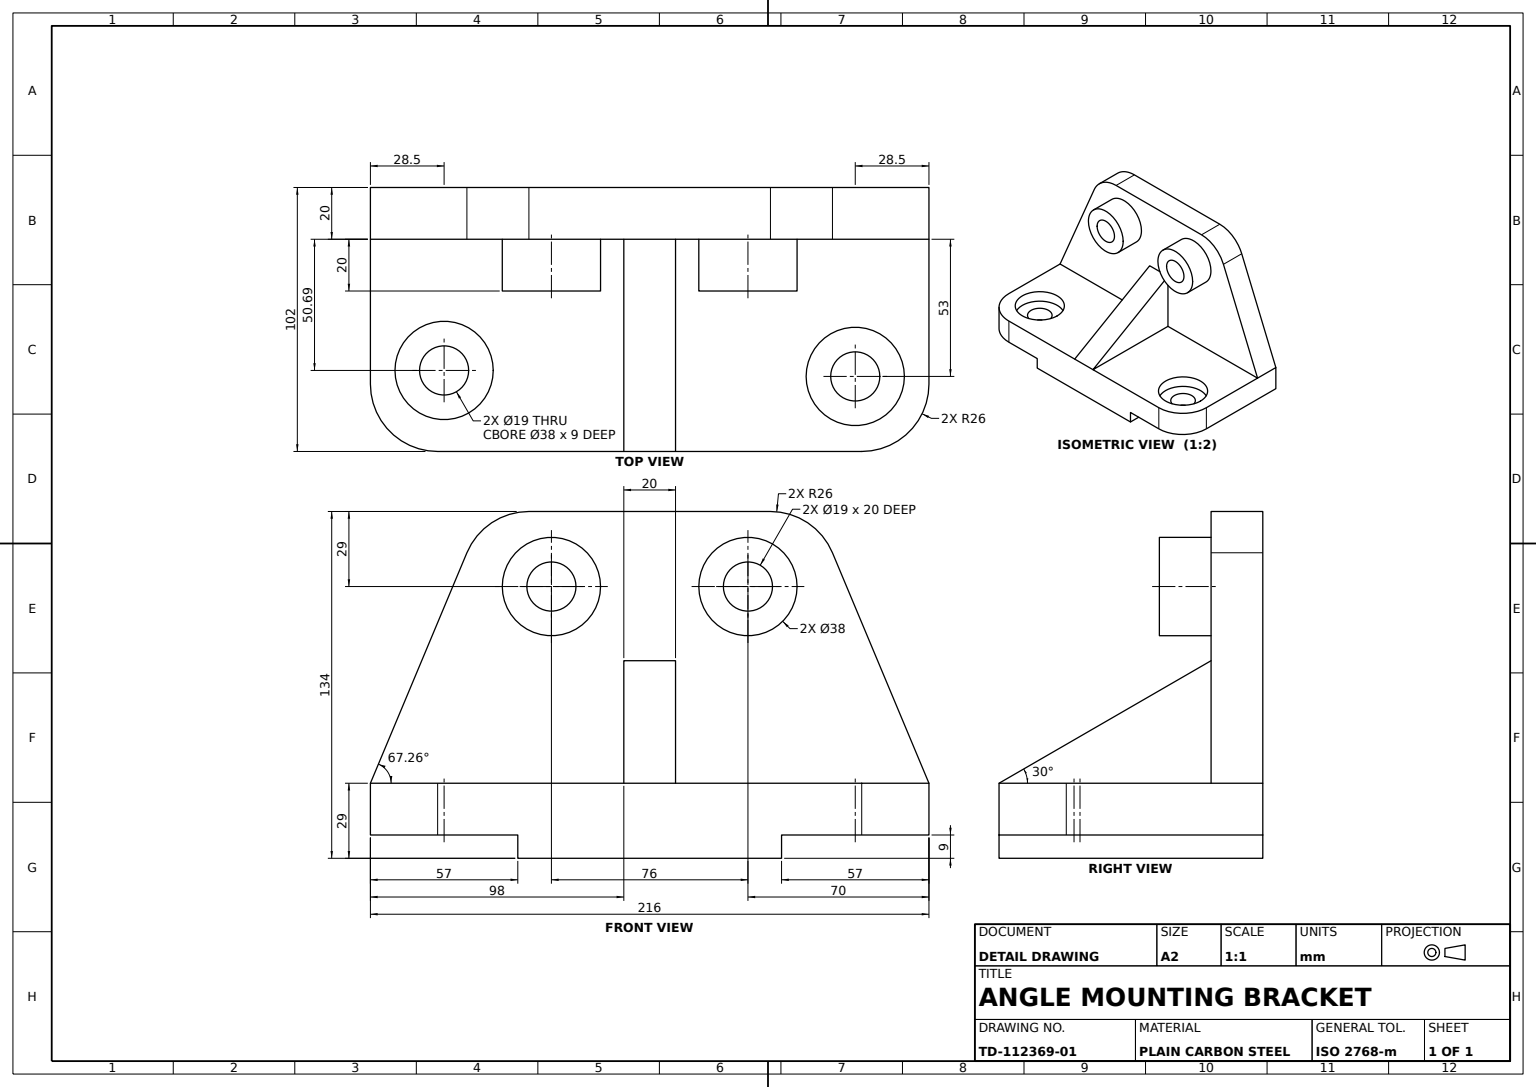
from build123d import *

# Parameters (mm, degrees)
BASE_PLATE_DEPTH                = 102
UPRIGHT_PLATE_DEPTH             = 20
UPRIGHT_BOSS_1_PROFILE_R        = 19
UPRIGHT_BOSS_1_PROFILE_R_2      = 9.5
UPRIGHT_BOSS_1_DEPTH            = 20
UPRIGHT_BOSS_2_PROFILE_R        = 19
UPRIGHT_BOSS_2_PROFILE_R_2      = 9.5
UPRIGHT_BOSS_2_DEPTH            = 20
BASE_POCKET_1_PROFILE_R         = 19
BASE_POCKET_1_DEPTH             = 9
MOUNTING_HOLE_1_PROFILE_R       = 9.5
MOUNTING_HOLE_1_DEPTH           = 265.680940001
BASE_POCKET_2_PROFILE_R         = 19
BASE_POCKET_2_DEPTH             = 9
MOUNTING_HOLE_2_PROFILE_R       = 9.5
MOUNTING_HOLE_2_DEPTH           = 265.680940001
UPRIGHT_CORNER_FILLET_R26_1_R   = 26
UPRIGHT_CORNER_FILLET_R26_2_R   = 26
BASE_CORNER_FILLETS_R26_R       = 26
GUSSET_RIB_REACH                = 196.147
GUSSET_RIB_PROFILE_30DEG_WALL_W = 484.979147418
GUSSET_RIB_PROFILE_30DEG_WALL_H = 20


with BuildPart() as part:
    # Base Plate Profile → Base Plate (new body)
    with BuildSketch(Plane(origin=(0, 0, 0), x_dir=(0, 0, -1), z_dir=(1, 0, 0))):
        Polygon((0, 0), (57, 0), (57, -9), (159, -9), (159, 0), (216, 0), (216, 20), (0, 20), align=None)
    extrude(amount=BASE_PLATE_DEPTH)

    # Upright Plate Profile → Upright Plate (add)
    with BuildSketch(Plane(origin=(0, 0, 0), x_dir=(0, 0, -1), z_dir=(1, 0, 0))):
        Polygon((0, 20), (216, 20), (172, 125), (44, 125), align=None)
    extrude(amount=UPRIGHT_PLATE_DEPTH)

    # Upright Boss 1 Profile → Upright Boss 1 (add)
    with BuildSketch(Plane(origin=(20, 0, 0), x_dir=(0, 0, -1), z_dir=(1, 0, 0))):
        with Locations((70, 96)):
            Circle(UPRIGHT_BOSS_1_PROFILE_R)
        with Locations((70, 96)):
            Circle(UPRIGHT_BOSS_1_PROFILE_R_2, mode=Mode.SUBTRACT)
    extrude(amount=UPRIGHT_BOSS_1_DEPTH)

    # Upright Boss 2 Profile → Upright Boss 2 (add)
    with BuildSketch(Plane(origin=(20, 0, 0), x_dir=(0, 0, -1), z_dir=(1, 0, 0))):
        with Locations((146, 96)):
            Circle(UPRIGHT_BOSS_2_PROFILE_R)
        with Locations((146, 96)):
            Circle(UPRIGHT_BOSS_2_PROFILE_R_2, mode=Mode.SUBTRACT)
    extrude(amount=UPRIGHT_BOSS_2_DEPTH)

    # Base Pocket 1 Profile → Base Pocket 1 (cut)
    with BuildSketch(Plane(origin=(0, 20, 0), x_dir=(1, 0, 0), z_dir=(0, 1, 0))):
        with Locations(Location((73, 187.5, 0), (0, 0, 270))):
            Circle(BASE_POCKET_1_PROFILE_R)
    extrude(amount=-BASE_POCKET_1_DEPTH, mode=Mode.SUBTRACT)

    # Mounting Hole 1 Profile → Mounting Hole 1 (cut, through all)
    with BuildSketch(Plane(origin=(0, 11, 0), x_dir=(1, 0, 0), z_dir=(0, 1, 0))):
        with Locations(Location((73, 187.5, 0), (0, 0, 270))):
            Circle(MOUNTING_HOLE_1_PROFILE_R)
    extrude(amount=-MOUNTING_HOLE_1_DEPTH, mode=Mode.SUBTRACT)

    # Base Pocket 2 Profile → Base Pocket 2 (cut)
    with BuildSketch(Plane(origin=(0, 20, 0), x_dir=(1, 0, 0), z_dir=(0, 1, 0))):
        with Locations(Location((70.69, 28.5, 0), (0, 0, 270))):
            Circle(BASE_POCKET_2_PROFILE_R)
    extrude(amount=-BASE_POCKET_2_DEPTH, mode=Mode.SUBTRACT)

    # Mounting Hole 2 Profile → Mounting Hole 2 (cut, through all)
    with BuildSketch(Plane(origin=(0, 11, 0), x_dir=(1, 0, 0), z_dir=(0, 1, 0))):
        with Locations(Location((70.69, 28.5, 0), (0, 0, 270))):
            Circle(MOUNTING_HOLE_2_PROFILE_R)
    extrude(amount=-MOUNTING_HOLE_2_DEPTH, mode=Mode.SUBTRACT)

    # Upright Corner Fillet R26 1
    upright_corner_fillet_r26_1_edges = [part.edges().sort_by_distance(p)[0] for p in [
        (10, 125, -44),
    ]]
    fillet(upright_corner_fillet_r26_1_edges, radius=UPRIGHT_CORNER_FILLET_R26_1_R)

    # Upright Corner Fillet R26 2
    upright_corner_fillet_r26_2_edges = [part.edges().sort_by_distance(p)[0] for p in [
        (10, 125, -172),
    ]]
    fillet(upright_corner_fillet_r26_2_edges, radius=UPRIGHT_CORNER_FILLET_R26_2_R)

    # Base Corner Fillets R26
    base_corner_fillets_r26_edges = [part.edges().sort_by_distance(p)[0] for p in [
        (102, 10, -216),
        (102, 10, 0),
    ]]
    fillet(base_corner_fillets_r26_edges, radius=BASE_CORNER_FILLETS_R26_R)

    # Gusset Rib Profile 30deg wall → Gusset Rib (add, up to next)
    with BuildSketch(Plane(origin=(61, 43.671361037, -108), x_dir=(-0.866025403782, 0.500000000004, 0), z_dir=(-0.500000000004, -0.866025403782, 0)), mode=Mode.PRIVATE) as gusset_rib_sk1:
        Rectangle(GUSSET_RIB_PROFILE_30DEG_WALL_W, GUSSET_RIB_PROFILE_30DEG_WALL_H)
    gusset_rib_tool1 = extrude(gusset_rib_sk1.sketch, amount=GUSSET_RIB_REACH, mode=Mode.PRIVATE) - part.part
    add(gusset_rib_tool1.solids().sort_by_distance((61, 43.671361037, -108))[0])


solid = part.part
